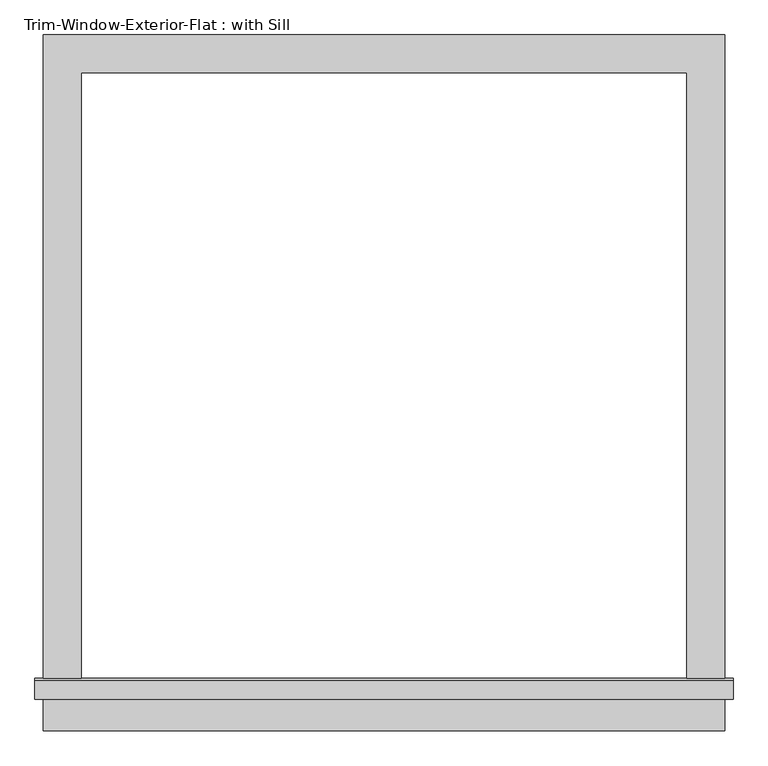
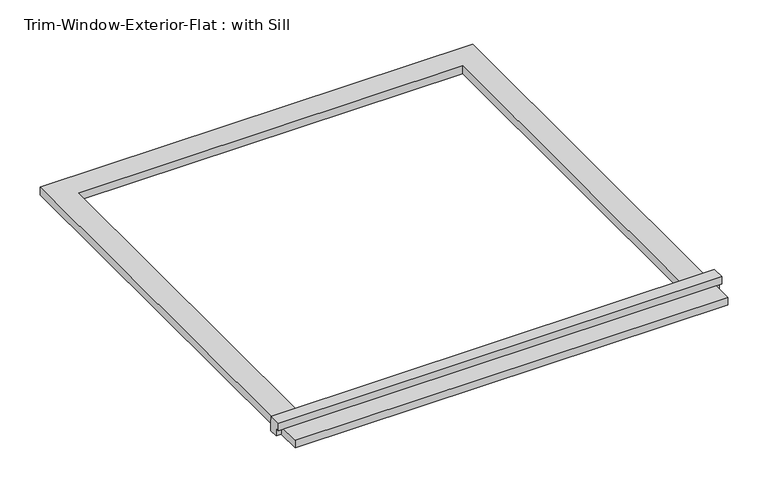
"""IFC4 building model written with IfcOpenShell, lengths in millimetres: proxy geometry, Trim-Window-Exterior-Flat : with Sill."""

from ifc_helpers import new_model, si_unit, frame, origin, origin_with_axes, place, context, project, spatial, polyline, outline, extrude, source, transform, mapped, element, save


def trim_window_exterior_flat_with_sill_84e24481(model_context):
    return source(origin(), model_context, "Body", "SweptSolid", [
        extrude(outline(polyline([(514.35, -936.5823709), (514.35, -993.7323709), (-514.35, -993.7323709), (-514.35, -936.5823709), (514.35, -936.5823709)])), origin_with_axes(), (0.0, 0.0, 1.0), 19.05),
        extrude(outline(polyline([(-946.15, 38.1), (-916.8580645, 38.1), (-914.4, 19.05), (-914.4, 0.0), (-936.5823709, 0.0), (-936.5823709, 19.05), (-946.15, 19.05), (-946.15, 38.1)])), frame((-527.05, 0.0, 0.0), z_axis=(1.0, 0.0, 0.0), x_axis=(0.0, 1.0, 0.0)), (0.0, 0.0, 1.0), 1054.1),
        extrude(outline(polyline([(-514.35, 57.15), (514.35, 57.15), (514.35, -914.4), (457.2, -914.4), (457.2, 0.0), (-457.2, 0.0), (-457.2, -914.4), (-514.35, -914.4), (-514.35, 57.15)])), origin_with_axes(), (0.0, 0.0, 1.0), 19.05),
    ])


if __name__ == "__main__":
    model = new_model("IFC4")
    model_context = context("Model", 3, world=origin())
    ifc_project = project(units=[si_unit("LENGTHUNIT", "METRE", prefix="MILLI")], contexts=[model_context])
    site = spatial("IfcSite", under=ifc_project)
    building = spatial("IfcBuilding", under=site)
    placement = place(None, origin())
    trim_window_exterior_flat_with_sill_shape = trim_window_exterior_flat_with_sill_84e24481(model_context)
    element("IfcBuildingElementProxy", 1, Name="Trim-Window-Exterior-Flat : with Sill", ObjectType="Trim-Window-Exterior-Flat : with Sill", at=placement, inside=building, context=model_context, shape_type="MappedRepresentation", body=[
        mapped(trim_window_exterior_flat_with_sill_shape, transform((0.0, 0.0, 0.0), x_axis=(1.0, 0.0, 0.0), y_axis=(0.0, 1.0, 0.0), z_axis=(0.0, 0.0, 1.0))),
    ])
    save(model, "model.ifc")

# Revit data of these elements
# Type "Trim-Window-Exterior-Flat : with Sill"
#   Trim Width = 0' - 2 1/4"
#   Trim Thickness_Picture Frame = 0' - 1 1/4"
#   Trim Thickness_with Sill = 0' - 0 3/4"
#   Sill Thickness = 0' - 1 1/4"
#   Opening Width [instance default] = 2' - 0"
#   Opening Height [instance default] = 3' - 0"
#   Default Elevation = 4' - 0"
#   Sill = yes
#   Picture Frame = no
#   Trim Material [instance default] = none
# Element 1 (IfcBuildingElementProxy, "Trim-Window-Exterior-Flat : with Sill")
#   Opening Width = 3' - 0"
